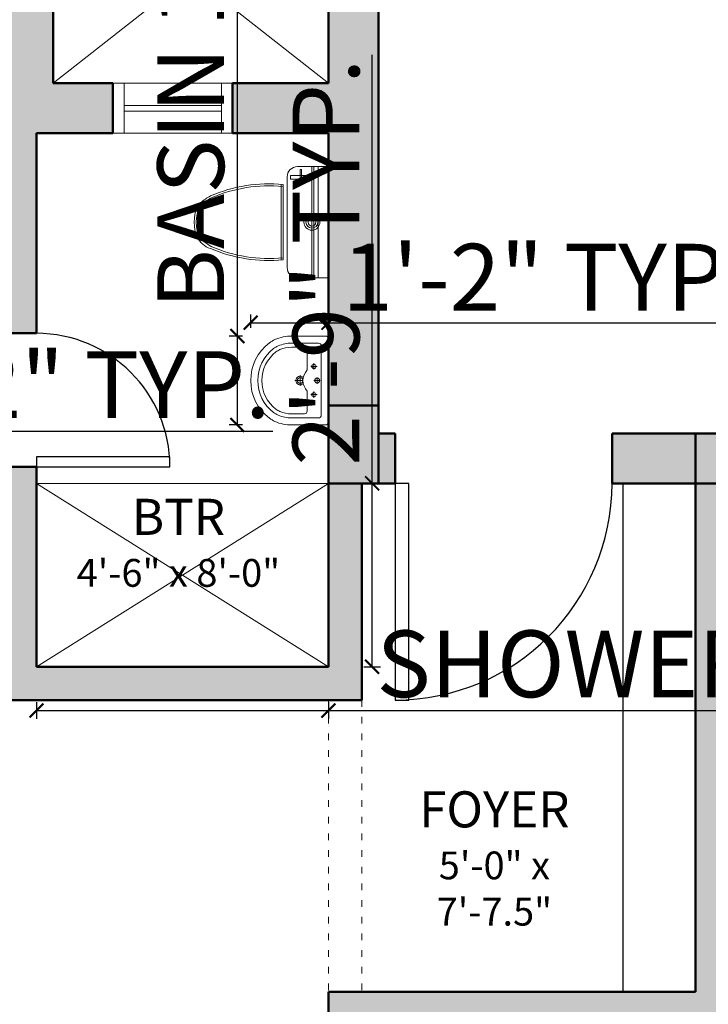
# Model space of a CAD drawing. Units: inches. Extents: x 375 to 1122, y 27 to 1069.
# Tile 78 of 155: x 667 to 790, y 400 to 577. Entities that reach past the tile are written whole.
import ezdxf

# ---------------------------------------------------------------- set-up
doc = ezdxf.new("R2010")
doc.units = ezdxf.units.IN
doc.linetypes.add('ACAD_ISO03W100', pattern=[30, 12, -18])
for name, color, linetype, lineweight in [('A-ANNO-DIMS', 2, 'Continuous', 18), ('A-AREA-IDEN', 7, 'Continuous', 18), ('A-COLS-PATT', 10, 'Continuous', 13), ('A-FLOR-FIXT', 55, 'Continuous', 18), ('A-FLOR-MILL', 55, 'Continuous', 25), ('A-FLOR-OPEN', 250, 'Continuous', 18), ('A-WALL-OVHD', 77, 'ACAD_ISO03W100', 18), ('A-WALL-PATT', 252, 'Continuous', 13), ('Columns', 10, 'Continuous', 50), ('Doors', 150, 'Continuous', 25), ('Shower Areas', 53, 'Continuous', 18), ('Walls', 250, 'Continuous', 50), ('Windows', 122, 'Continuous', 18)]:
    doc.layers.add(name, color=color, linetype=linetype, lineweight=lineweight)
doc.styles.get("Standard").update_dxf_attribs({"font": 'arial.ttf'})
doc.dimstyles.new('ISO-25', dxfattribs={"dimtxt": 12, "dimasz": 2.5, "dimexe": 1.5, "dimexo": 1.5, "dimtad": 1, "dimdec": 1, "dimlunit": 3, "dimtxsty": 'Standard', "dimblk": 'ARCHTICK', "dimcen": 2.5, "dimadec": 0, "dimazin": 0, "dimtfac": 1, "dimtdec": 1, "dimtmove": 0, "dimatfit": 3, "dimfxl": 1.5, "dimfxlon": 1, "dimarcsym": 0})

# ---------------------------------------------------------------- blocks, each defined once
blk = doc.blocks.new('*U5')
for p, q in [((0, 0), (0, 4)), ((28, 0), (28, 4))]:
    blk.add_line(p, q)
blk.add_lwpolyline([(0, 0), (0, -28), (1.75, -28), (1.75, 0)], close=True)
blk.add_arc((0, 0), 28, 270, 0)
blk = doc.blocks.new('*U11')
for p, q in [((-24, 0), (-24, -4)), ((0, 0), (0, -4))]:
    blk.add_line(p, q)
blk.add_lwpolyline([(0, 0), (0, 24), (-1.75, 24), (-1.75, 0)], close=True)
blk.add_arc((0, 0), 24, 90, 180)
blk = doc.blocks.new('A$C00C51FE0')
at = {"ltscale": 2}
for p, q in [((1.85, 7.41), (18.15, 7.41)), ((16.79, 8.49), (3.21, 8.49)), ((16.79, 8.12), (3.21, 8.12)), ((0, 0), (0, 5.56)), ((1.59, 4.18), (1.59, 6.81)), ((1.59, 6.81), (2.25, 6.81)), ((2.25, 6.81), (2.25, 4.18)), ((20, 5.56), (20, 0)), ((0.5, 4.84), (0.5, 5.06)), ((0.5, 5.06), (2.91, 5.06)), ((2.91, 4.84), (0.5, 4.84)), ((2.25, 4.18), (1.59, 4.18)), ((2.91, 5.06), (2.91, 4.84)), ((20, 2.96), (0, 2.96)), ((20, 2.59), (0, 2.59)), ((20, 1.85), (0, 1.85)), ((20, 0), (0, 0))]:
    blk.add_line(p, q, dxfattribs=at)
for radius in [1.44, 1.07, 0.698]:
    blk.add_circle((10, 2.96), radius, dxfattribs=at)
for centre, radius, start, end in [((22.68, 10.69), 19.97, 141.7352, 148.8373), ((7.96, 21.86), 1.85, 112.9199, 142.816), ((10, 17.03), 6.73, 63.5839, 116.4161), ((10, 17.03), 7.1, 67.0801, 112.9199), ((11.04, 20.15), 3.83, 16.1902, 63.2078), ((-2.68, 10.69), 19.97, 31.1627, 38.2648), ((22.68, 10.69), 20.34, 142.816, 148.8373), ((29.69, 10.65), 26.6, 156.5869, 185.4494), ((29.69, 10.65), 26.23, 156.5869, 185.4494), ((-9.69, 10.65), 26.23, 354.5506, 23.4131), ((-9.69, 10.65), 26.6, 354.5506, 23.4131), ((1.85, 5.56), 1.85, 90, 180), ((18.15, 5.56), 1.85, 0, 90)]:
    blk.add_arc(centre, radius, start, end, dxfattribs=at)
blk = doc.blocks.new('WINDOW-21_5IN')
for p, q in [((4, 2), (4, 19.5)), ((5, 2), (5, 19.5))]:
    blk.add_line(p, q)
blk.add_lwpolyline([(0, 0), (9, 0), (9, 21.5), (0, 21.5)], close=True)
for points in [[(9, 19.5), (0, 19.5)], [(0, 2), (9, 2)]]:
    blk.add_lwpolyline(points)
blk = doc.blocks.new('LAVATORY-16IN')
for p, q in [((1.78, 12.7), (14.22, 12.7)), ((8, 11.37), (8, 12.51)), ((1.27, 7.37), (1.27, 12.19)), ((4.89, 11.37), (6.03, 11.37)), ((5.46, 10.79), (5.46, 11.94)), ((7.43, 11.94), (8.57, 11.94)), ((9.97, 11.37), (11.11, 11.37)), ((10.54, 10.79), (10.54, 11.94)), ((14.73, 12.19), (14.73, 7.37)), ((2.01, 7.37), (2.01, 9.65)), ((2.51, 10.16), (6.08, 10.16)), ((7.02, 8.89), (8.98, 8.89)), ((8, 7.91), (8, 9.4)), ((9.91, 10.16), (13.49, 10.16)), ((13.99, 9.65), (13.99, 7.37))]:
    blk.add_line(p, q)
blk.add_lwpolyline([(0.51, 13.97), (15.49, 13.97, -0.414214), (16, 13.46), (16, 7.37, -0.104704), (15.37, 4.36, -0.038376), (14.78, 3.36, -0.495903), (1.22, 3.36, -0.038376), (0.63, 4.36, -0.104704), (0, 7.37), (0, 13.46, -0.414214)], format="xyb", close=True)
for points in [[(1.27, 7.37, 0.102694), (1.78, 4.92, 0.037256), (2.25, 4.11, 0.085618)], [(2.01, 7.37, 0.101044), (2.44, 5.24, 0.036381), (2.84, 4.54, 0.084644)], [(13.16, 4.54, 0.036381), (13.56, 5.24, 0.101044), (13.99, 7.37, 0.11083)], [(13.75, 4.11, 0.037256), (14.22, 4.92, 0.102694), (14.73, 7.37, 0.111333)]]:
    blk.add_lwpolyline(points, format="xyb")
for centre, radius in [((5.46, 11.37), 0.381), ((8, 11.94), 0.444), ((10.54, 11.37), 0.381), ((8, 8.89), 0.508)]:
    blk.add_circle(centre, radius)
for centre, radius, start, end in [((1.78, 12.19), 0.508, 90, 180), ((14.22, 12.19), 0.508, 0, 90), ((2.51, 9.65), 0.508, 90, 180), ((7.99, 12.19), 2.79, 226.6581, 313.3419), ((8, 8.89), 0.762, 133.135, 47.0367), ((13.49, 9.65), 0.508, 0, 90), ((8, 8.52), 7.25, 217.471, 322.529), ((8, 8.52), 6.51, 217.6433, 322.3567)]:
    blk.add_arc(centre, radius, start, end)
blk = doc.blocks.new('COLUMN-14X9IN')
blk.add_lwpolyline([(0, 0), (14, 0), (14, 9), (0, 9)], close=True)
blk = doc.blocks.new('SHOWER-PAN-52_5X33IN')
for p, q in [((0, 33), (52.5, 0)), ((52.5, 33), (0, 0))]:
    blk.add_line(p, q)
blk.add_lwpolyline([(0, 0), (52.5, 0), (52.5, 33), (0, 33)], close=True)
blk = doc.blocks.new('_ArchTick')
at = {"color": 0, "linetype": 'ByBlock', "const_width": 0.15}
blk.add_lwpolyline([(-0.5, -0.5), (0.5, 0.5)], dxfattribs=at)
blk = doc.blocks.new('*D44')
at = {"layer": 'A-ANNO-DIMS', "color": 0, "lineweight": -2, "transparency": 16777216}
for p, q in [((541.85, 504.43), (541.85, 501.43)), ((607.16, 504.43), (607.16, 501.43)), ((541.85, 502.93), (607.16, 502.93)), ((607.16, 502.93), (712.02, 502.93))]:
    blk.add_line(p, q, dxfattribs=at)
at = {"layer": 'Defpoints', "color": 0, "transparency": 16777216}
for p in [(541.85, 513.06), (607.16, 513.06), (607.16, 502.93)]:
    blk.add_point(p, dxfattribs=at)
at = {"layer": 'A-ANNO-DIMS', "color": 0, "lineweight": -2, "transparency": 16777216, "xscale": 2.5, "yscale": 2.5, "zscale": 2.5, "rotation": 180}
blk.add_blockref('_ArchTick', (541.85, 502.93), dxfattribs=at)
at = {"layer": 'A-ANNO-DIMS', "color": 0, "lineweight": -2, "transparency": 16777216, "xscale": 2.5, "yscale": 2.5, "zscale": 2.5}
blk.add_blockref('_ArchTick', (607.16, 502.93), dxfattribs=at)
at = {"layer": 'A-ANNO-DIMS', "color": 0, "transparency": 16777216, "insert": (660.84, 509.76), "char_height": 12, "attachment_point": 5}
blk.add_mtext('5\'-5 1/2" TYP.', dxfattribs=at)
blk = doc.blocks.new('*D51')
at = {"layer": 'A-ANNO-DIMS', "color": 0, "lineweight": -2, "transparency": 16777216}
for p, q in [((705.64, 520.03), (705.64, 651.36)), ((706.54, 520.03), (704.14, 520.03)), ((705.64, 504.03), (705.64, 520.03)), ((706.54, 504.03), (704.14, 504.03))]:
    blk.add_line(p, q, dxfattribs=at)
at = {"layer": 'Defpoints', "color": 0, "transparency": 16777216}
for p in [(705.64, 520.03), (708.04, 520.03), (708.04, 504.03)]:
    blk.add_point(p, dxfattribs=at)
at = {"layer": 'A-ANNO-DIMS', "color": 0, "lineweight": -2, "transparency": 16777216, "xscale": 2.5, "yscale": 2.5, "zscale": 2.5}
for p, rotation in [((705.64, 520.03), 90), ((705.64, 504.03), 270)]:
    blk.add_blockref('_ArchTick', p, dxfattribs=dict(at, rotation=rotation))
at = {"layer": 'A-ANNO-DIMS', "color": 0, "transparency": 16777216, "insert": (698.81, 586.94), "char_height": 12, "attachment_point": 5, "rotation": 90}
blk.add_mtext('BASIN 1\'-4" TYP.', dxfattribs=at)
blk = doc.blocks.new('*D52')
at = {"layer": 'A-ANNO-DIMS', "color": 0, "lineweight": -2, "transparency": 16777216}
for p, q in [((708.04, 521.53), (708.04, 523.93)), ((722.01, 521.53), (722.01, 523.93)), ((708.04, 522.43), (722.01, 522.43)), ((722.01, 522.43), (797.77, 522.43))]:
    blk.add_line(p, q, dxfattribs=at)
at = {"layer": 'Defpoints', "color": 0, "transparency": 16777216}
for p in [(722.01, 522.43), (708.04, 520.03), (722.01, 520.03)]:
    blk.add_point(p, dxfattribs=at)
at = {"layer": 'A-ANNO-DIMS', "color": 0, "lineweight": -2, "transparency": 16777216, "xscale": 2.5, "yscale": 2.5, "zscale": 2.5, "rotation": 180}
blk.add_blockref('_ArchTick', (708.04, 522.43), dxfattribs=at)
at = {"layer": 'A-ANNO-DIMS', "color": 0, "lineweight": -2, "transparency": 16777216, "xscale": 2.5, "yscale": 2.5, "zscale": 2.5}
blk.add_blockref('_ArchTick', (722.01, 522.43), dxfattribs=at)
at = {"layer": 'A-ANNO-DIMS', "color": 0, "transparency": 16777216, "insert": (761.14, 529.08), "char_height": 12, "attachment_point": 5}
blk.add_mtext('1\'-2" TYP.', dxfattribs=at)
blk = doc.blocks.new('*D53')
at = {"layer": 'A-ANNO-DIMS', "color": 0, "lineweight": -2, "transparency": 16777216}
for p, q in [((669.51, 454.15), (669.51, 451.15)), ((722.01, 454.15), (722.01, 451.15)), ((669.51, 452.65), (722.01, 452.65)), ((722.01, 452.65), (946.03, 452.65))]:
    blk.add_line(p, q, dxfattribs=at)
at = {"layer": 'Defpoints', "color": 0, "transparency": 16777216}
for p in [(669.51, 460.53), (722.01, 460.53), (722.01, 452.65)]:
    blk.add_point(p, dxfattribs=at)
at = {"layer": 'A-ANNO-DIMS', "color": 0, "lineweight": -2, "transparency": 16777216, "xscale": 2.5, "yscale": 2.5, "zscale": 2.5, "rotation": 180}
blk.add_blockref('_ArchTick', (669.51, 452.65), dxfattribs=at)
at = {"layer": 'A-ANNO-DIMS', "color": 0, "lineweight": -2, "transparency": 16777216, "xscale": 2.5, "yscale": 2.5, "zscale": 2.5}
blk.add_blockref('_ArchTick', (722.01, 452.65), dxfattribs=at)
at = {"layer": 'A-ANNO-DIMS', "color": 0, "transparency": 16777216, "insert": (835.27, 459.49), "char_height": 12, "attachment_point": 5}
blk.add_mtext('SHOWER PAN 4\'-4 1/2" TYP.', dxfattribs=at)
blk = doc.blocks.new('*D54')
at = {"layer": 'A-ANNO-DIMS', "color": 0, "lineweight": -2, "transparency": 16777216}
for p, q in [((729.88, 493.53), (729.88, 570.63)), ((728.38, 493.53), (731.38, 493.53)), ((729.88, 460.53), (729.88, 493.53)), ((728.38, 460.53), (731.38, 460.53))]:
    blk.add_line(p, q, dxfattribs=at)
at = {"layer": 'Defpoints', "color": 0, "transparency": 16777216}
for p in [(722.01, 493.53), (729.88, 493.53), (722.01, 460.53)]:
    blk.add_point(p, dxfattribs=at)
at = {"layer": 'A-ANNO-DIMS', "color": 0, "lineweight": -2, "transparency": 16777216, "xscale": 2.5, "yscale": 2.5, "zscale": 2.5}
for p, rotation in [((729.88, 493.53), 90), ((729.88, 460.53), 270)]:
    blk.add_blockref('_ArchTick', p, dxfattribs=dict(at, rotation=rotation))
at = {"layer": 'A-ANNO-DIMS', "color": 0, "transparency": 16777216, "insert": (723.13, 533.33), "char_height": 12, "attachment_point": 5, "rotation": 90}
blk.add_mtext('2\'-9" TYP.', dxfattribs=at)
blk = doc.blocks.new('*D80')
at = {"layer": 'A-ANNO-DIMS', "color": 0, "lineweight": -2, "transparency": 16777216}
for p, q in [((641.51, 582.33), (641.51, 579.33)), ((663.51, 582.33), (663.51, 579.33)), ((641.51, 580.83), (663.51, 580.83)), ((663.51, 580.83), (748.6, 580.83))]:
    blk.add_line(p, q, dxfattribs=at)
at = {"layer": 'Defpoints', "color": 0, "transparency": 16777216}
for p in [(641.51, 589.53), (663.51, 589.53), (663.51, 580.83)]:
    blk.add_point(p, dxfattribs=at)
at = {"layer": 'A-ANNO-DIMS', "color": 0, "lineweight": -2, "transparency": 16777216, "xscale": 2.5, "yscale": 2.5, "zscale": 2.5, "rotation": 180}
blk.add_blockref('_ArchTick', (641.51, 580.83), dxfattribs=at)
at = {"layer": 'A-ANNO-DIMS', "color": 0, "lineweight": -2, "transparency": 16777216, "xscale": 2.5, "yscale": 2.5, "zscale": 2.5}
blk.add_blockref('_ArchTick', (663.51, 580.83), dxfattribs=at)
at = {"layer": 'A-ANNO-DIMS', "color": 0, "transparency": 16777216, "insert": (707.3, 587.58), "char_height": 12, "attachment_point": 5}
blk.add_mtext('1\'-10" TYP.', dxfattribs=at)
blk = doc.blocks.new('*D88')
at = {"layer": 'A-ANNO-DIMS', "color": 0, "lineweight": -2, "transparency": 16777216}
for p, q in [((731.01, 1052.53), (731.01, 1055.53)), ((854.01, 1052.53), (854.01, 1055.53)), ((731.01, 1054.03), (854.01, 1054.03))]:
    blk.add_line(p, q, dxfattribs=at)
at = {"layer": 'Defpoints', "color": 0, "transparency": 16777216}
for p in [(854.01, 1054.03), (731.01, 502.53), (854.01, 502.53)]:
    blk.add_point(p, dxfattribs=at)
at = {"layer": 'A-ANNO-DIMS', "color": 0, "lineweight": -2, "transparency": 16777216, "xscale": 2.5, "yscale": 2.5, "zscale": 2.5, "rotation": 180}
blk.add_blockref('_ArchTick', (731.01, 1054.03), dxfattribs=at)
at = {"layer": 'A-ANNO-DIMS', "color": 0, "lineweight": -2, "transparency": 16777216, "xscale": 2.5, "yscale": 2.5, "zscale": 2.5}
blk.add_blockref('_ArchTick', (854.01, 1054.03), dxfattribs=at)
at = {"layer": 'A-ANNO-DIMS', "color": 0, "transparency": 16777216, "insert": (792.51, 1060.78), "char_height": 12, "attachment_point": 5}
blk.add_mtext('10\'-3"', dxfattribs=at)
blk = doc.blocks.new('*D90')
at = {"layer": 'A-ANNO-DIMS', "color": 0, "lineweight": -2, "transparency": 16777216}
for p, q in [((401.51, 574.53), (398.51, 574.53)), ((400.01, 502.53), (400.01, 574.53)), ((401.51, 502.53), (398.51, 502.53))]:
    blk.add_line(p, q, dxfattribs=at)
at = {"layer": 'Defpoints', "color": 0, "transparency": 16777216}
for p in [(400.01, 574.53), (863.01, 574.53), (863.01, 502.53)]:
    blk.add_point(p, dxfattribs=at)
at = {"layer": 'A-ANNO-DIMS', "color": 0, "lineweight": -2, "transparency": 16777216, "xscale": 2.5, "yscale": 2.5, "zscale": 2.5}
for p, rotation in [((400.01, 574.53), 90), ((400.01, 502.53), 270)]:
    blk.add_blockref('_ArchTick', p, dxfattribs=dict(at, rotation=rotation))
at = {"layer": 'A-ANNO-DIMS', "color": 0, "transparency": 16777216, "insert": (393.26, 538.53), "char_height": 12, "attachment_point": 5, "rotation": 90}
blk.add_mtext('6\'-0"', dxfattribs=at)
blk = doc.blocks.new('*D94')
at = {"layer": 'A-ANNO-DIMS', "color": 0, "lineweight": -2, "transparency": 16777216}
for p, q in [((734.01, 117.53), (734.01, 114.53)), ((773.01, 117.53), (773.01, 114.53)), ((734.01, 116.03), (773.01, 116.03))]:
    blk.add_line(p, q, dxfattribs=at)
at = {"layer": 'Defpoints', "color": 0, "transparency": 16777216}
for p in [(734.01, 667.53), (773.01, 667.53), (773.01, 116.03)]:
    blk.add_point(p, dxfattribs=at)
at = {"layer": 'A-ANNO-DIMS', "color": 0, "lineweight": -2, "transparency": 16777216, "xscale": 2.5, "yscale": 2.5, "zscale": 2.5, "rotation": 180}
blk.add_blockref('_ArchTick', (734.01, 116.03), dxfattribs=at)
at = {"layer": 'A-ANNO-DIMS', "color": 0, "lineweight": -2, "transparency": 16777216, "xscale": 2.5, "yscale": 2.5, "zscale": 2.5}
blk.add_blockref('_ArchTick', (773.01, 116.03), dxfattribs=at)
at = {"layer": 'A-ANNO-DIMS', "color": 0, "transparency": 16777216, "insert": (753.51, 122.78), "char_height": 12, "attachment_point": 5}
blk.add_mtext('3\'-3"', dxfattribs=at)

msp = doc.modelspace()

# ---------------------------------------------------------------- hatches: boundary and pattern name
at = {"layer": 'A-COLS-PATT'}
h = msp.add_hatch(color=256, dxfattribs=at)
h.dxf.hatch_style = 1
h.paths.add_polyline_path([(512.51, 982.53), (498.51, 982.53), (498.51, 973.53), (512.51, 973.53)])
h.paths.add_polyline_path([(666.51, 982.53), (652.51, 982.53), (652.51, 973.53), (666.51, 973.53)])
h.paths.add_polyline_path([(802.01, 982.53), (788.01, 982.53), (788.01, 973.53), (802.01, 973.53)])
h.paths.add_polyline_path([(932.01, 982.53), (918.01, 982.53), (918.01, 973.53), (932.01, 973.53)])
h.paths.add_polyline_path([(507.51, 841.53), (498.51, 841.53), (498.51, 827.53), (507.51, 827.53)])
h.paths.add_polyline_path([(666.51, 844.53), (652.51, 844.53), (652.51, 835.53), (666.51, 835.53)])
h.paths.add_polyline_path([(802.01, 814.53), (788.01, 814.53), (788.01, 805.53), (802.01, 805.53)])
h.paths.add_polyline_path([(932.01, 814.53), (918.01, 814.53), (918.01, 805.53), (932.01, 805.53)])
h.paths.add_polyline_path([(507.51, 719.53), (498.51, 719.53), (498.51, 705.53), (507.51, 705.53)])
h.paths.add_polyline_path([(731.01, 676.53), (722.01, 676.53), (722.01, 662.53), (731.01, 662.53)])
h.paths.add_polyline_path([(802.01, 676.53), (788.01, 676.53), (788.01, 667.53), (802.01, 667.53)])
h.paths.add_polyline_path([(932.01, 676.53), (918.01, 676.53), (918.01, 667.53), (932.01, 667.53)])
h.paths.add_polyline_path([(932.01, 583.53), (918.01, 583.53), (918.01, 574.53), (932.01, 574.53)])
h.paths.add_polyline_path([(868.01, 583.53), (854.01, 583.53), (854.01, 574.53), (868.01, 574.53)])
h.paths.add_polyline_path([(868.01, 502.53), (854.01, 502.53), (854.01, 493.53), (868.01, 493.53)])
h.paths.add_polyline_path([(932.01, 502.53), (918.01, 502.53), (918.01, 493.53), (932.01, 493.53)])
h.paths.add_polyline_path([(672.51, 592.03), (663.51, 592.03), (663.51, 578.03), (672.51, 578.03)])
h.paths.add_polyline_path([(512.51, 589.53), (498.51, 589.53), (498.51, 580.53), (512.51, 580.53)])
h.paths.add_polyline_path([(507.51, 464.53), (498.51, 464.53), (498.51, 450.53), (507.51, 450.53)])
h.paths.add_polyline_path([(731.01, 507.53), (722.01, 507.53), (722.01, 493.53), (731.01, 493.53)])
h.paths.add_polyline_path([(802.01, 502.53), (788.01, 502.53), (788.01, 493.53), (802.01, 493.53)])
h.paths.add_polyline_path([(507.51, 342.53), (498.51, 342.53), (498.51, 328.53), (507.51, 328.53)])
h.paths.add_polyline_path([(512.51, 196.53), (498.51, 196.53), (498.51, 187.53), (512.51, 187.53)])
h.paths.add_polyline_path([(666.51, 334.53), (652.51, 334.53), (652.51, 325.53), (666.51, 325.53)])
h.paths.add_polyline_path([(666.51, 196.53), (652.51, 196.53), (652.51, 187.53), (666.51, 187.53)])
h.paths.add_polyline_path([(805.01, 196.53), (791.01, 196.53), (791.01, 187.53), (805.01, 187.53)])
h.paths.add_polyline_path([(932.01, 196.53), (918.01, 196.53), (918.01, 187.53), (932.01, 187.53)])
h.paths.add_polyline_path([(932.01, 334.53), (918.01, 334.53), (918.01, 325.53), (932.01, 325.53)])
h.paths.add_polyline_path([(805.01, 334.53), (791.01, 334.53), (791.01, 325.53), (805.01, 325.53)])
at = {"layer": 'A-WALL-PATT'}
h = msp.add_hatch(color=256, dxfattribs=at)
h.dxf.hatch_style = 1
h.paths.add_polyline_path([(962.01, 388.53), (989.01, 388.53), (989.01, 394.53), (962.01, 394.53), (932.01, 394.53), (932.01, 397.53), (923.01, 397.53), (923.01, 394.53), (842.01, 394.53), (842.01, 334.53), (839.51, 334.53), (839.51, 328.53), (854.01, 328.53), (854.01, 334.53), (848.01, 334.53), (848.01, 388.53), (953.01, 388.53), (953.01, 356.08), (962.01, 356.08), (962.01, 358.55), (989.01, 358.55), (989.01, 364.55), (962.01, 364.55)])
h.paths.add_polyline_path([(989.01, 502.53), (932.01, 502.53), (932.01, 583.53), (932.01, 593.53), (923.01, 593.53), (923.01, 583.53), (854.01, 583.53), (854.01, 556.53), (863.01, 556.53), (863.01, 574.53), (923.01, 574.53), (923.01, 502.53), (863.01, 502.53), (863.01, 520.53), (854.01, 520.53), (854.01, 502.53), (773.01, 502.53), (773.01, 493.53), (788.01, 493.53), (788.01, 402.03), (722.01, 402.03), (722.01, 373.53), (728.01, 373.53), (728.01, 396.03), (788.01, 396.03), (788.01, 373.53), (794.01, 373.53), (794.01, 430.53), (814.01, 430.53), (814.01, 436.53), (794.01, 436.53), (794.01, 493.53), (923.01, 493.53), (923.01, 487.53), (932.01, 487.53), (932.01, 493.53), (983.01, 493.53), (983.01, 473.53), (989.01, 473.53)])
h.paths.add_polyline_path([(797.01, 325.53), (805.01, 325.53), (805.01, 328.53), (807.51, 328.53), (807.51, 334.53), (791.01, 334.53), (791.01, 226.53), (770.76, 226.53), (770.76, 217.53), (791.01, 217.53), (791.01, 187.53), (855.01, 187.53), (855.01, 196.53), (797.01, 196.53)])
h.paths.add_polyline_path([(989.01, 238.53), (962.01, 238.53), (962.01, 256.42), (953.01, 256.42), (953.01, 229.53), (980.01, 229.53), (980.01, 196.53), (915.01, 196.53), (915.01, 187.53), (989.01, 187.53)])
h.paths.add_polyline_path([(962.01, 334.53), (884.01, 334.53), (884.01, 328.53), (918.01, 328.53), (918.01, 325.53), (932.01, 325.53), (932.01, 328.53), (953.01, 328.53), (953.01, 304.42), (962.01, 304.42)])
h.paths.add_polyline_path([(606.51, 283.53), (609.51, 283.53), (609.51, 289.53), (600.51, 289.53), (600.51, 196.53), (578.51, 196.53), (578.51, 187.53), (606.51, 187.53), (606.51, 196.53)])
h.paths.add_polyline_path([(666.51, 292.53), (660.51, 292.53), (660.51, 289.53), (633.51, 289.53), (633.51, 283.53), (660.51, 283.53), (660.51, 196.53), (628.01, 196.53), (628.01, 187.53), (630.53, 187.53), (630.53, 160.53), (636.53, 160.53), (636.53, 187.53), (660.51, 187.53), (660.51, 160.53), (666.51, 160.53), (666.51, 217.53), (686.76, 217.53), (686.76, 226.53), (666.51, 226.53)])
h.paths.add_polyline_path([(480.51, 256.42), (471.51, 256.42), (471.51, 238.53), (444.51, 238.53), (444.51, 187.53), (518.51, 187.53), (518.51, 196.53), (453.51, 196.53), (453.51, 229.53), (480.51, 229.53)])
h.paths.add_polyline_path([(480.51, 328.53), (652.51, 328.53), (652.51, 325.53), (660.51, 325.53), (660.51, 322.53), (666.51, 322.53), (666.51, 334.53), (507.51, 334.53), (507.51, 360.53), (498.51, 360.53), (498.51, 334.53), (471.51, 334.53), (471.51, 304.42), (480.51, 304.42)])
h.paths.add_polyline_path([(507.51, 484.53), (498.51, 484.53), (498.51, 444.53), (507.51, 444.53), (507.51, 454.53), (621.51, 454.53), (621.51, 460.53), (507.51, 460.53)])
h.paths.add_polyline_path([(672.51, 604.53), (683.26, 604.53), (683.26, 613.53), (669.51, 613.53), (669.51, 649.53), (663.51, 649.53), (663.51, 589.53), (507.51, 589.53), (507.51, 613.53), (498.51, 613.53), (498.51, 556.53), (507.51, 556.53), (507.51, 580.53), (663.51, 580.53), (663.51, 520.53), (669.51, 520.53), (669.51, 556.53), (683.26, 556.53), (683.26, 565.53), (672.51, 565.53)])
h.paths.add_polyline_path([(731.01, 667.53), (734.01, 667.53), (734.01, 676.53), (728.01, 676.53), (728.01, 715.53), (657.51, 715.53), (657.51, 709.53), (663.51, 709.53), (663.51, 673.53), (669.51, 673.53), (669.51, 709.53), (722.01, 709.53), (722.01, 613.53), (704.76, 613.53), (704.76, 604.53), (722.01, 604.53), (722.01, 565.53), (704.76, 565.53), (704.76, 556.53), (722.01, 556.53), (722.01, 502.53), (722.01, 460.53), (669.51, 460.53), (669.51, 496.53), (663.51, 496.53), (663.51, 460.53), (657.51, 460.53), (657.51, 454.53), (728.01, 454.53), (728.01, 493.53), (734.01, 493.53), (734.01, 502.53), (731.01, 502.53)])
h.paths.add_polyline_path([(986.01, 718.53), (959.01, 718.53), (959.01, 727.53), (950.01, 727.53), (950.01, 709.53), (977.01, 709.53), (977.01, 676.53), (794.01, 676.53), (794.01, 805.53), (802.01, 805.53), (802.01, 808.53), (804.51, 808.53), (804.51, 814.53), (788.01, 814.53), (788.01, 774.03), (728.01, 774.03), (728.01, 796.53), (722.01, 796.53), (722.01, 768.03), (788.01, 768.03), (788.01, 676.53), (773.01, 676.53), (773.01, 667.53), (923.01, 667.53), (923.01, 657.53), (932.01, 657.53), (932.01, 667.53), (986.01, 667.53)])
h.paths.add_polyline_path([(621.51, 715.53), (507.51, 715.53), (507.51, 733.53), (498.51, 733.53), (498.51, 715.53), (498.51, 685.53), (507.51, 685.53), (507.51, 709.53), (621.51, 709.53)])
h.paths.add_polyline_path([(666.51, 847.03), (660.51, 847.03), (660.51, 844.53), (652.51, 844.53), (652.51, 841.53), (480.51, 841.53), (480.51, 859.53), (471.51, 859.53), (471.51, 835.53), (498.51, 835.53), (498.51, 817.53), (507.51, 817.53), (507.51, 835.53), (666.51, 835.53)])
h.paths.add_polyline_path([(480.51, 940.53), (453.51, 940.53), (453.51, 973.53), (518.51, 973.53), (518.51, 982.53), (444.51, 982.53), (444.51, 931.53), (471.51, 931.53), (471.51, 907.53), (480.51, 907.53)])
h.paths.add_polyline_path([(606.51, 982.53), (578.51, 982.53), (578.51, 973.53), (600.51, 973.53), (600.51, 880.53), (609.51, 880.53), (609.51, 886.53), (606.51, 886.53)])
h.paths.add_polyline_path([(666.51, 943.53), (686.76, 943.53), (686.76, 952.53), (666.51, 952.53), (666.51, 1009.53), (660.51, 1009.53), (660.51, 982.53), (636.53, 982.53), (636.53, 1009.53), (630.53, 1009.53), (630.53, 982.53), (628.01, 982.53), (628.01, 973.53), (660.51, 973.53), (660.51, 886.53), (633.51, 886.53), (633.51, 880.53), (660.51, 880.53), (660.51, 877.03), (666.51, 877.03)])
h.paths.add_polyline_path([(986.01, 874.53), (932.01, 874.53), (932.01, 877.53), (923.01, 877.53), (923.01, 874.53), (788.01, 874.53), (788.01, 868.53), (788.01, 844.53), (794.01, 844.53), (794.01, 868.53), (839.01, 868.53), (839.01, 814.53), (836.51, 814.53), (836.51, 808.53), (851.01, 808.53), (851.01, 814.53), (845.01, 814.53), (845.01, 868.53), (986.01, 868.53)])
h.paths.add_polyline_path([(959.01, 838.55), (986.01, 838.55), (986.01, 844.55), (959.01, 844.55), (959.01, 847.03), (950.01, 847.03), (950.01, 814.53), (881.01, 814.53), (881.01, 808.53), (918.01, 808.53), (918.01, 805.53), (932.01, 805.53), (932.01, 808.53), (950.01, 808.53), (950.01, 793.53), (959.01, 793.53)])
h.paths.add_polyline_path([(986.01, 982.53), (899.01, 982.53), (899.01, 973.53), (923.01, 973.53), (923.01, 967.53), (932.01, 967.53), (932.01, 973.53), (980.01, 973.53), (980.01, 953.53), (986.01, 953.53)])
h.paths.add_polyline_path([(851.01, 982.53), (788.01, 982.53), (788.01, 952.53), (770.76, 952.53), (770.76, 943.53), (788.01, 943.53), (788.01, 910.53), (814.01, 910.53), (814.01, 916.53), (794.01, 916.53), (794.01, 973.53), (851.01, 973.53)])

# ---------------------------------------------------------------- linework, layer by layer
at = {"layer": 'A-FLOR-MILL'}
msp.add_line((775.01, 402.03), (775.01, 493.53), dxfattribs=at)
at = {"layer": 'A-FLOR-OPEN'}
for p, q in [((672.51, 604.53), (722.01, 565.53)), ((722.01, 604.53), (672.51, 565.53))]:
    msp.add_line(p, q, dxfattribs=at)
at = {"layer": 'A-WALL-OVHD', "ltscale": 0.1}
for p, q in [((722.01, 454.53), (722.01, 402.03)), ((728.01, 454.53), (728.01, 402.03))]:
    msp.add_line(p, q, dxfattribs=at)
at = {"layer": 'Walls'}
for p, q in [((731.01, 502.53), (731.01, 667.53)), ((672.51, 565.53), (672.51, 604.53)), ((722.01, 565.53), (722.01, 604.53)), ((672.51, 565.53), (683.26, 565.53)), ((683.26, 565.53), (683.26, 556.53)), ((704.76, 565.53), (704.76, 556.53)), ((704.76, 565.53), (722.01, 565.53)), ((669.51, 556.53), (683.26, 556.53)), ((669.51, 520.53), (669.51, 556.53)), ((704.76, 556.53), (722.01, 556.53)), ((722.01, 502.53), (722.01, 556.53)), ((669.51, 520.53), (663.51, 520.53)), ((722.01, 460.53), (722.01, 502.53)), ((734.01, 502.53), (731.01, 502.53)), ((734.01, 502.53), (734.01, 493.53)), ((773.01, 502.53), (773.01, 493.53)), ((854.01, 502.53), (773.01, 502.53)), ((669.51, 496.53), (663.51, 496.53)), ((669.51, 460.53), (669.51, 496.53)), ((728.01, 454.53), (728.01, 493.53)), ((734.01, 493.53), (728.01, 493.53)), ((788.01, 493.53), (773.01, 493.53)), ((788.01, 402.03), (788.01, 493.53)), ((669.51, 460.53), (722.01, 460.53)), ((657.51, 454.53), (728.01, 454.53)), ((722.01, 373.53), (722.01, 402.03)), ((788.01, 402.03), (722.01, 402.03))]:
    msp.add_line(p, q, dxfattribs=at)

# ---------------------------------------------------------------- block references
at = {"layer": 'A-FLOR-FIXT', "xscale": -1, "rotation": 90}
msp.add_blockref('A$C00C51FE0', (722.01, 550.53), dxfattribs=at)
at = {"layer": 'A-FLOR-FIXT', "extrusion": (0, 0, -1), "zscale": -1, "rotation": 90}
msp.add_blockref('LAVATORY-16IN', (-708.04, 504.03), dxfattribs=at)
at = {"layer": 'Columns', "extrusion": (0, 0, -1), "zscale": -1, "rotation": 270}
msp.add_blockref('COLUMN-14X9IN', (-731.01, 507.53), dxfattribs=at)
at = {"layer": 'Columns', "extrusion": (0, 0, -1), "zscale": -1}
msp.add_blockref('COLUMN-14X9IN', (-802.01, 493.53), dxfattribs=at)
at = {"layer": 'Doors', "rotation": 270}
msp.add_blockref('*U11', (669.51, 496.53), dxfattribs=at)
at = {"layer": 'Doors', "xscale": 1.392857142857142, "yscale": 1.392857142857142, "zscale": 1.392857142857142}
msp.add_blockref('*U5', (734.01, 493.53), dxfattribs=at)
at = {"layer": 'Shower Areas'}
msp.add_blockref('SHOWER-PAN-52_5X33IN', (669.51, 460.53), dxfattribs=at)
at = {"layer": 'Windows', "rotation": 90}
msp.add_blockref('WINDOW-21_5IN', (704.76, 556.53), dxfattribs=at)

# ---------------------------------------------------------------- texts
at = {"layer": 'A-AREA-IDEN', "char_height": 6.5, "attachment_point": 1}
for s, insert in [('\\pxqc;{\\fArial|b1|i0|c0|p34;BTR\\P\\fArial|b0|i0|c0|p34;\\H0.76923x;4\'-6" x 8\'-0"}', (673.93, 490.75)), ('\\pxqc;{\\fArial|b1|i0|c0|p34;FOYER\\P\\fArial|b0|i0|c0|p34;\\H0.76923x;5\'-0" x 7\'-7.5"}', (730.74, 438.11))]:
    msp.add_mtext_dynamic_manual_height_columns(s, width=42.2291, gutter_width=12.5, heights=[0], dxfattribs=dict(at, insert=insert))

# ---------------------------------------------------------------- dimensions: what is measured, and where the dimension line sits
at = {"layer": 'A-ANNO-DIMS'}
for base, p1, p2, picture, middle in [((854.01, 1054.03), (731.01, 502.53), (854.01, 502.53), '*D88', (792.51, 1060.78)), ((773.01, 116.03), (734.01, 667.53), (773.01, 667.53), '*D94', (753.51, 122.78))]:
    dim = msp.add_linear_dim(base=base, p1=p1, p2=p2, dimstyle='ISO-25', override={"dimdec": 1, "dimlfac": 1, "dimrnd": 0, "dimzin": 1, "dimdsep": 46, "dimlunit": 4, "dimfrac": 2}, dxfattribs=at)
    dim.commit()
    dim.dimension.update_dxf_attribs({"geometry": picture, "text_midpoint": middle})
for base, p1, p2, text, picture, middle in [((705.64, 520.03), (708.04, 504.03), (708.04, 520.03), 'BASIN <> TYP.', '*D51', (698.81, 586.94)), ((729.88, 493.53), (722.01, 460.53), (722.01, 493.53), '<> TYP.', '*D54', (723.13, 533.33))]:
    dim = msp.add_linear_dim(base=base, p1=p1, p2=p2, angle=90, text=text, dimstyle='ISO-25', override={"dimdec": 1, "dimlfac": 1, "dimrnd": 0, "dimzin": 1, "dimdsep": 46, "dimlunit": 4, "dimfrac": 2}, dxfattribs=at)
    dim.commit()
    dim.dimension.update_dxf_attribs({"geometry": picture, "text_midpoint": middle})
for base, p1, p2, text, picture, middle in [((663.51, 580.83), (641.51, 589.53), (663.51, 589.53), '<> TYP.', '*D80', (707.3, 587.58)), ((722.01, 522.43), (708.04, 520.03), (722.01, 520.03), '<> TYP.', '*D52', (761.14, 529.08)), ((607.16, 502.93), (541.85, 513.06), (607.16, 513.06), '<> TYP.', '*D44', (660.84, 509.76)), ((722.01, 452.65), (669.51, 460.53), (722.01, 460.53), 'SHOWER PAN <> TYP.', '*D53', (835.27, 459.49))]:
    dim = msp.add_linear_dim(base=base, p1=p1, p2=p2, text=text, dimstyle='ISO-25', override={"dimdec": 1, "dimlfac": 1, "dimrnd": 0, "dimzin": 1, "dimdsep": 46, "dimlunit": 4, "dimfrac": 2}, dxfattribs=at)
    dim.commit()
    dim.dimension.update_dxf_attribs({"geometry": picture, "text_midpoint": middle})
dim = msp.add_linear_dim(base=(400.01, 574.53), p1=(863.01, 502.53), p2=(863.01, 574.53), angle=90, dimstyle='ISO-25', override={"dimdec": 1, "dimlfac": 1, "dimrnd": 0, "dimzin": 1, "dimdsep": 46, "dimlunit": 4, "dimfrac": 2}, dxfattribs=at)
dim.commit()
dim.dimension.update_dxf_attribs({"geometry": '*D90', "text_midpoint": (393.26, 538.53)})

doc.saveas('drawing.dxf')
